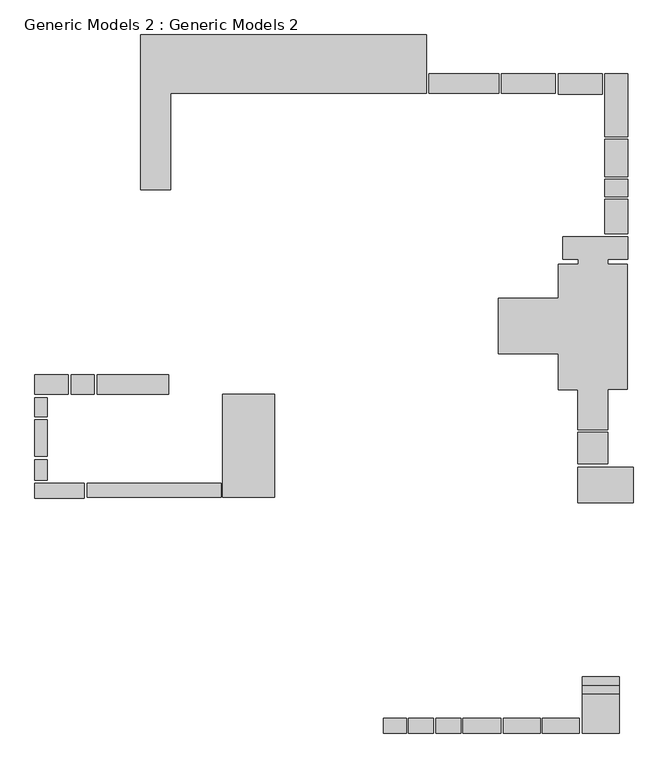
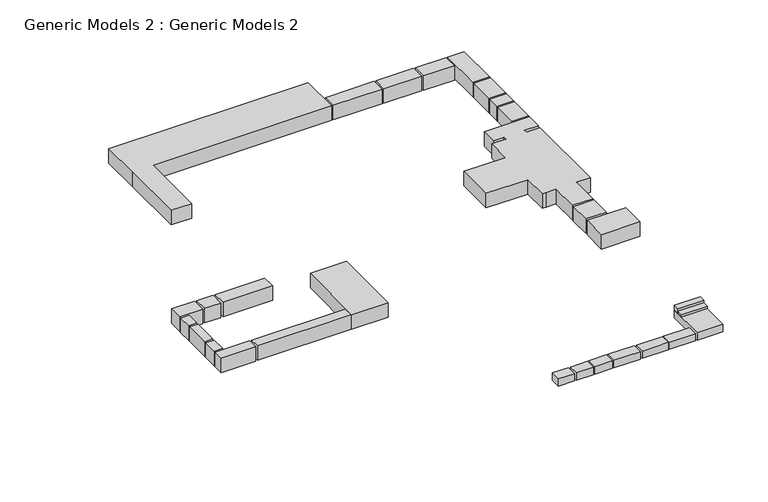
"""IFC4 building model written with IfcOpenShell, lengths in millimetres: proxy geometry, Generic Models 2 : Generic Models 2."""

from ifc_helpers import new_model, si_unit, frame, origin, place, context, project, spatial, polyline, outline, extrude, source, transform, mapped, element, save


def generic_models_2_generic_models_2_cbc3407a(model_context):
    return source(origin(), model_context, "Body", "SweptSolid", [
        extrude(outline(polyline([(1247.2588295, -11853.9978125), (328.8323081, -11853.9978125), (328.8323081, -11255.2794723), (1247.2588295, -11255.2794723), (1247.2588295, -11853.9978125)])), frame((0.0, 0.0, -914.4), z_axis=(0.0, 0.0, 1.0), x_axis=(1.0, 0.0, 0.0)), (0.0, 0.0, 1.0), 448.3109329),
        extrude(outline(polyline([(-11658.3527951, -1839.8731969), (-11658.3527951, -2449.4731969), (-13639.5527951, -2449.4731969), (-13639.5527951, -1839.8731969), (-11658.3527951, -1839.8731969)])), frame((0.0, 0.0, -914.4), z_axis=(0.0, 0.0, 1.0), x_axis=(1.0, 0.0, 0.0)), (0.0, 0.0, 1.0), 880.1109329),
        extrude(outline(polyline([(-11537.1113256, -2411.8945725), (-11537.1113256, -1839.8731969), (-6168.6851385, -1839.8731969), (-6168.6851385, -2411.8945725), (-11537.1113256, -2411.8945725)])), frame((0.0, 0.0, -914.4), z_axis=(0.0, 0.0, 1.0), x_axis=(1.0, 0.0, 0.0)), (0.0, 0.0, 1.0), 880.1109329),
        extrude(outline(polyline([(-6115.035762, -2411.8945725), (-6115.035762, 1710.0401753), (-4032.235762, 1710.0401753), (-4032.235762, -2411.8945725), (-6115.035762, -2411.8945725)])), frame((0.0, 0.0, -914.4), z_axis=(0.0, 0.0, 1.0), x_axis=(1.0, 0.0, 0.0)), (0.0, 0.0, 1.0), 880.1109329),
        extrude(outline(polyline([(-11136.5794247, 2491.7950806), (-8287.6635431, 2491.7950806), (-8287.6635431, 1710.0401753), (-11136.5794247, 1710.0401753), (-11136.5794247, 2491.7950806)])), frame((0.0, 0.0, -914.4), z_axis=(0.0, 0.0, 1.0), x_axis=(1.0, 0.0, 0.0)), (0.0, 0.0, 1.0), 880.1109329),
        extrude(outline(polyline([(-12189.2966097, 2491.7950806), (-11261.5895905, 2491.7950806), (-11261.5895905, 1710.0401753), (-12189.2966097, 1710.0401753), (-12189.2966097, 2491.7950806)])), frame((0.0, 0.0, -914.4), z_axis=(0.0, 0.0, 1.0), x_axis=(1.0, 0.0, 0.0)), (0.0, 0.0, 1.0), 880.1109329),
        extrude(outline(polyline([(-13636.7827389, 2491.7950806), (-12304.4375518, 2491.7950806), (-12304.4375518, 1710.0401753), (-13636.7827389, 1710.0401753), (-13636.7827389, 2491.7950806)])), frame((0.0, 0.0, -914.4), z_axis=(0.0, 0.0, 1.0), x_axis=(1.0, 0.0, 0.0)), (0.0, 0.0, 1.0), 880.1109329),
        extrude(outline(polyline([(-13154.1827389, 1583.8265087), (-13154.1827389, 821.8265087), (-13636.7827389, 821.8265087), (-13636.7827389, 1583.8265087), (-13154.1827389, 1583.8265087)])), frame((0.0, 0.0, -914.4), z_axis=(0.0, 0.0, 1.0), x_axis=(1.0, 0.0, 0.0)), (0.0, 0.0, 1.0), 880.1109329),
        extrude(outline(polyline([(-13154.1827389, 702.1758663), (-13154.1827389, -768.3384514), (-13636.7827389, -768.3384514), (-13636.7827389, 702.1758663), (-13154.1827389, 702.1758663)])), frame((0.0, 0.0, -914.4), z_axis=(0.0, 0.0, 1.0), x_axis=(1.0, 0.0, 0.0)), (0.0, 0.0, 1.0), 880.1109329),
        extrude(outline(polyline([(-13154.1827389, -909.7973231), (-13154.1827389, -1722.3634002), (-13636.7827389, -1722.3634002), (-13636.7827389, -909.7973231), (-13154.1827389, -909.7973231)])), frame((0.0, 0.0, -914.4), z_axis=(0.0, 0.0, 1.0), x_axis=(1.0, 0.0, 0.0)), (0.0, 0.0, 1.0), 880.1109329),
        extrude(outline(polyline([(7337.4638577, 5556.2586043), (7337.4638577, 6926.196618), (8137.7595608, 6926.196618), (8137.7595608, 7129.396618), (7528.1595608, 7129.396618), (7528.1595608, 8018.396618), (10131.6595608, 8018.396618), (10131.6595608, 7129.396618), (9318.8595608, 7129.396618), (9318.8595608, 6926.196618), (10106.2595608, 6926.196618), (10106.2595608, 1922.396618), (9318.8595608, 1922.396618), (9318.8595608, 296.796618), (8125.0595608, 296.796618), (8125.0595608, 1903.346618), (7541.4179176, 1903.346618), (7336.8310303, 1903.346618), (7336.8310303, 3345.1052847), (4936.5310303, 3345.1052847), (4936.5310303, 5556.2586043), (7337.4638577, 5556.2586043)])), frame((0.0, 0.0, -914.4), z_axis=(0.0, 0.0, 1.0), x_axis=(1.0, 0.0, 0.0)), (0.0, 0.0, 1.0), 880.1109329),
        extrude(outline(polyline([(10334.8595608, -2623.3351307), (8125.0595608, -2623.3351307), (8125.0595608, -1200.9351307), (10334.8595608, -1200.9351307), (10334.8595608, -2623.3351307)])), frame((0.0, 0.0, -914.4), z_axis=(0.0, 0.0, 1.0), x_axis=(1.0, 0.0, 0.0)), (0.0, 0.0, 1.0), 880.1109329),
        extrude(outline(polyline([(9318.8595608, -1059.0936581), (8125.0595608, -1059.0936581), (8125.0595608, 185.5063419), (9318.8595608, 185.5063419), (9318.8595608, -1059.0936581)])), frame((0.0, 0.0, -914.4), z_axis=(0.0, 0.0, 1.0), x_axis=(1.0, 0.0, 0.0)), (0.0, 0.0, 1.0), 880.1109329),
        extrude(outline(polyline([(9191.8595608, 8135.0104025), (9191.8595608, 9532.0104025), (10131.6595608, 9532.0104025), (10131.6595608, 8135.0104025), (9191.8595608, 8135.0104025)])), frame((0.0, 0.0, -914.4), z_axis=(0.0, 0.0, 1.0), x_axis=(1.0, 0.0, 0.0)), (0.0, 0.0, 1.0), 880.1109329),
        extrude(outline(polyline([(9191.8595608, 9628.5529086), (9191.8595608, 10322.6883024), (10131.6595608, 10322.6883024), (10131.6595608, 9628.5529086), (9191.8595608, 9628.5529086)])), frame((0.0, 0.0, -914.4), z_axis=(0.0, 0.0, 1.0), x_axis=(1.0, 0.0, 0.0)), (0.0, 0.0, 1.0), 880.1109329),
        extrude(outline(polyline([(9191.8595608, 10431.2497621), (9191.8595608, 11921.502527), (10131.6595608, 11921.502527), (10131.6595608, 10431.2497621), (9191.8595608, 10431.2497621)])), frame((0.0, 0.0, -914.4), z_axis=(0.0, 0.0, 1.0), x_axis=(1.0, 0.0, 0.0)), (0.0, 0.0, 1.0), 880.1109329),
        extrude(outline(polyline([(9191.8595608, 12030.0639867), (9191.8595608, 14544.6639867), (10131.6595608, 14544.6639867), (10131.6595608, 12030.0639867), (9191.8595608, 12030.0639867)])), frame((0.0, 0.0, -914.4), z_axis=(0.0, 0.0, 1.0), x_axis=(1.0, 0.0, 0.0)), (0.0, 0.0, 1.0), 880.1109329),
        extrude(outline(polyline([(7336.8310303, 14544.6639867), (9102.9498688, 14544.6639867), (9102.9498688, 13722.5893019), (7336.8310303, 13722.5893019), (7336.8310303, 14544.6639867)])), frame((0.0, 0.0, -914.4), z_axis=(0.0, 0.0, 1.0), x_axis=(1.0, 0.0, 0.0)), (0.0, 0.0, 1.0), 880.1109329),
        extrude(outline(polyline([(5066.1141474, 14544.6639867), (7229.3286758, 14544.6639867), (7229.3286758, 13770.1951007), (5066.1141474, 13770.1951007), (5066.1141474, 14544.6639867)])), frame((0.0, 0.0, -914.4), z_axis=(0.0, 0.0, 1.0), x_axis=(1.0, 0.0, 0.0)), (0.0, 0.0, 1.0), 880.1109329),
        extrude(outline(polyline([(2159.9892262, 14544.6639867), (4959.1509173, 14544.6639867), (4959.1509173, 13770.1951007), (2159.9892262, 13770.1951007), (2159.9892262, 14544.6639867)])), frame((0.0, 0.0, -914.4), z_axis=(0.0, 0.0, 1.0), x_axis=(1.0, 0.0, 0.0)), (0.0, 0.0, 1.0), 880.1109329),
        extrude(outline(polyline([(-8197.835762, 13770.1951007), (-8197.835762, 9909.3951007), (-9393.7178012, 9909.3951007), (-9393.7178012, 13770.1951007), (-9393.7178012, 16106.9951007), (2061.6821988, 16106.9951007), (2061.6821988, 13770.1951007), (-8197.835762, 13770.1951007)])), frame((0.0, 0.0, -914.4), z_axis=(0.0, 0.0, 1.0), x_axis=(1.0, 0.0, 0.0)), (0.0, 0.0, 1.0), 880.1109329),
        extrude(outline(polyline([(9781.6588295, -9934.1151761), (9781.6588295, -10276.6508799), (8295.7588295, -10276.6508799), (8295.7588295, -9934.1151761), (9781.6588295, -9934.1151761)])), frame((0.0, 0.0, -466.0890671), z_axis=(0.0, 0.0, 1.0), x_axis=(1.0, 0.0, 0.0)), (0.0, 0.0, 1.0), 152.4),
        extrude(outline(polyline([(9781.6588295, -9591.5794723), (9781.6588295, -9934.1151761), (8295.7588295, -9934.1151761), (8295.7588295, -9591.5794723), (9781.6588295, -9591.5794723)])), frame((0.0, 0.0, -466.0890671), z_axis=(0.0, 0.0, 1.0), x_axis=(1.0, 0.0, 0.0)), (0.0, 0.0, 1.0), 304.8),
        extrude(outline(polyline([(9781.6588295, -11853.9978125), (8295.7588295, -11853.9978125), (8295.7588295, -9591.5794723), (9781.6588295, -9591.5794723), (9781.6588295, -11853.9978125)])), frame((0.0, 0.0, -914.4), z_axis=(0.0, 0.0, 1.0), x_axis=(1.0, 0.0, 0.0)), (0.0, 0.0, 1.0), 448.3109329),
        extrude(outline(polyline([(8181.4588295, -11853.9978125), (6708.2588295, -11853.9978125), (6708.2588295, -11255.2794723), (8181.4588295, -11255.2794723), (8181.4588295, -11853.9978125)])), frame((0.0, 0.0, -914.4), z_axis=(0.0, 0.0, 1.0), x_axis=(1.0, 0.0, 0.0)), (0.0, 0.0, 1.0), 448.3109329),
        extrude(outline(polyline([(6627.0179176, -11853.9978125), (5133.4588295, -11853.9978125), (5133.4588295, -11255.2794723), (6627.0179176, -11255.2794723), (6627.0179176, -11853.9978125)])), frame((0.0, 0.0, -914.4), z_axis=(0.0, 0.0, 1.0), x_axis=(1.0, 0.0, 0.0)), (0.0, 0.0, 1.0), 448.3109329),
        extrude(outline(polyline([(5031.8588295, -11853.9978125), (3507.8588295, -11853.9978125), (3507.8588295, -11255.2794723), (5031.8588295, -11255.2794723), (5031.8588295, -11853.9978125)])), frame((0.0, 0.0, -914.4), z_axis=(0.0, 0.0, 1.0), x_axis=(1.0, 0.0, 0.0)), (0.0, 0.0, 1.0), 448.3109329),
        extrude(outline(polyline([(3426.6179176, -11853.9978125), (2428.3390133, -11853.9978125), (2428.3390133, -11255.2794723), (3426.6179176, -11255.2794723), (3426.6179176, -11853.9978125)])), frame((0.0, 0.0, -914.4), z_axis=(0.0, 0.0, 1.0), x_axis=(1.0, 0.0, 0.0)), (0.0, 0.0, 1.0), 448.3109329),
        extrude(outline(polyline([(2339.4588295, -11853.9978125), (1338.1576597, -11853.9978125), (1338.1576597, -11255.2794723), (2339.4588295, -11255.2794723), (2339.4588295, -11853.9978125)])), frame((0.0, 0.0, -914.4), z_axis=(0.0, 0.0, 1.0), x_axis=(1.0, 0.0, 0.0)), (0.0, 0.0, 1.0), 448.3109329),
    ])


if __name__ == "__main__":
    model = new_model("IFC4")
    model_context = context("Model", 3, world=origin())
    ifc_project = project(units=[si_unit("LENGTHUNIT", "METRE", prefix="MILLI")], contexts=[model_context])
    site = spatial("IfcSite", under=ifc_project)
    building = spatial("IfcBuilding", under=site)
    placement = place(None, origin())
    generic_models_2_generic_models_2_shape = generic_models_2_generic_models_2_cbc3407a(model_context)
    element("IfcBuildingElementProxy", 1, Name="Generic Models 2 : Generic Models 2", ObjectType="Generic Models 2 : Generic Models 2", at=placement, inside=building, context=model_context, shape_type="MappedRepresentation", body=[
        mapped(generic_models_2_generic_models_2_shape, transform((0.0, 0.0, 0.0), x_axis=(1.0, 0.0, 0.0), y_axis=(0.0, 1.0, 0.0), z_axis=(0.0, 0.0, 1.0))),
    ])
    save(model, "model.ifc")
